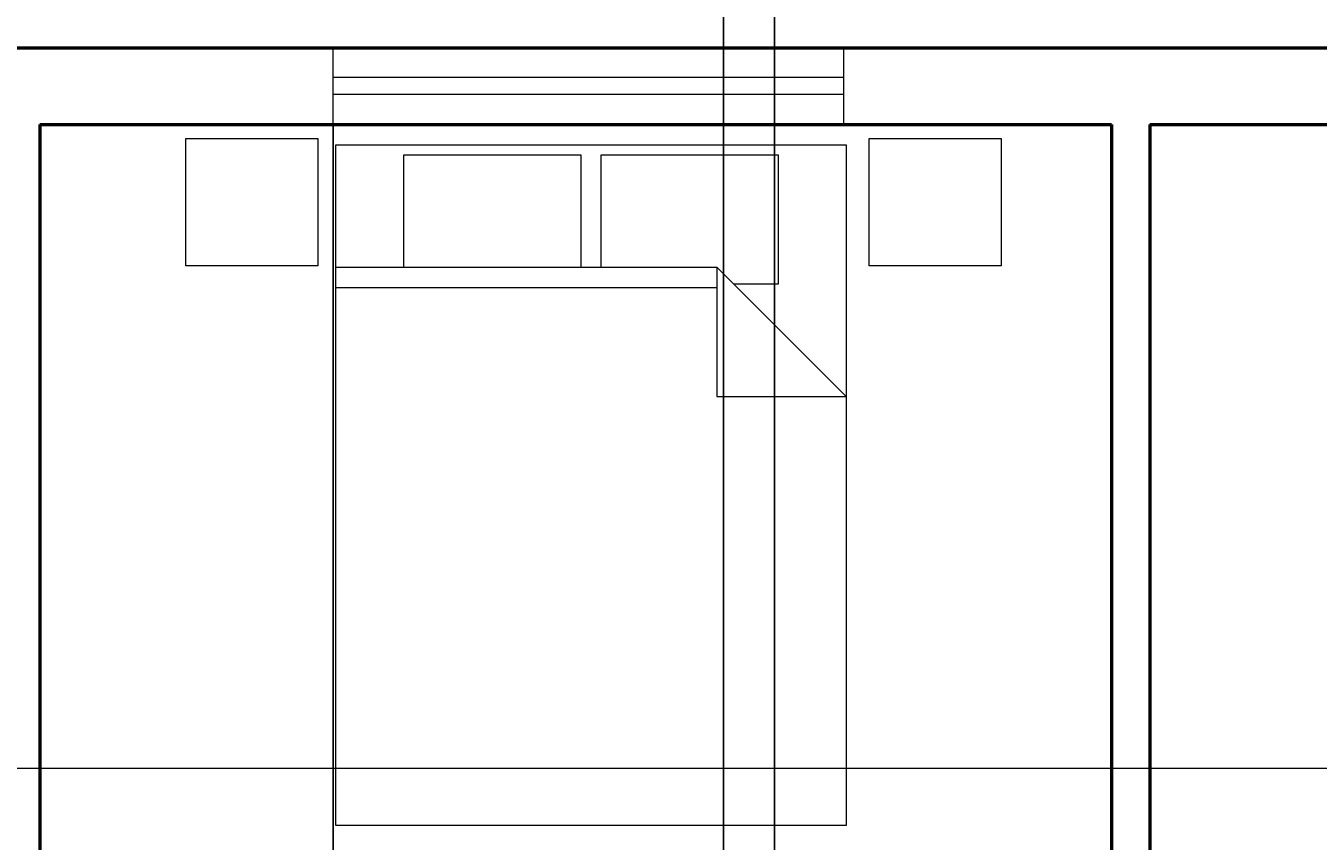
# Model space of a CAD drawing. Units: inches. Extents: x 7359 to 7979, y 33027 to 34263.
# Tile 16 of 32: x 7612 to 7764, y 33534 to 33630. Entities that reach past the tile are written whole.
import ezdxf

# ---------------------------------------------------------------- set-up
doc = ezdxf.new("R2010")
doc.units = ezdxf.units.IN
for name, color, linetype, lineweight in [('A-ANNO-DIMS', 2, 'Continuous', 18), ('A-ANNO-SYMB', 7, 'Continuous', 18), ('A-FURN', 8, 'Continuous', 18), ('A-GLAZ', 4, 'Continuous', 18), ('A-WALL', 7, 'Continuous', 50)]:
    doc.layers.add(name, color=color, linetype=linetype, lineweight=lineweight)
doc.styles.get("Standard").update_dxf_attribs({"font": 'arial.ttf'})
doc.dimstyles.get("Standard").update_dxf_attribs({"dimtxt": 0.18, "dimasz": 0.18, "dimexe": 0.18, "dimexo": 0.0625, "dimgap": 0.09, "dimtad": 0, "dimtih": 1, "dimtoh": 1, "dimdec": 4, "dimzin": 0, "dimdsep": 46, "dimtxsty": 'Standard', "dimcen": 0.09, "dimadec": 0, "dimazin": 0, "dimtfac": 1, "dimtdec": 4, "dimtofl": 0, "dimtmove": 0, "dimatfit": 3, "dimfxl": 1, "dimtolj": 1, "dimtzin": 0, "dimarcsym": 0})

# ---------------------------------------------------------------- blocks, each defined once
blk = doc.blocks.new('Bed - Queen')
for p, q in [((0, -80.00003), (0, 0)), ((0, 0), (59.99999, 0)), ((59.99999, 0), (59.99999, -80.00003)), ((7.99999, -1.2), (28.79998, -1.2)), ((7.99999, -14.4), (7.99999, -1.2)), ((28.79998, -1.2), (28.79998, -14.4)), ((31.19999, -1.2), (51.99999, -1.2)), ((31.19999, -14.4), (31.19999, -1.2)), ((51.99999, -1.2), (51.99999, -16.4)), ((0, -14.4), (44.8, -14.4)), ((59.99999, -29.6), (44.8, -14.4)), ((44.8, -14.4), (44.8, -29.6)), ((51.99999, -16.4), (46.79936, -16.4)), ((44.8, -16.8), (0, -16.8)), ((44.8, -29.6), (59.99999, -29.6)), ((59.99999, -80.00003), (0, -80.00003))]:
    blk.add_line(p, q)
blk = doc.blocks.new('TABLE-BEDSIDE')
blk.add_lwpolyline([(0, 15), (15.54, 15), (15.54, 0), (0, 0)], close=True)
blk = doc.blocks.new('WINDOW-W2-BEDROOM')
for p, q in [((0, 0), (0, 9)), ((60.05, 0), (60.05, 9)), ((60.05, 5.5), (0, 5.5)), ((60.05, 3.5), (0, 3.5))]:
    blk.add_line(p, q)
blk = doc.blocks.new('*D66')
at = {"layer": 'A-ANNO-DIMS', "color": 0, "lineweight": -2, "transparency": 16777216}
for p, q in [((7468.73, 33627.22), (7468.73, 33657.24)), ((7468.91, 33657.06), (7681.03, 33657.06)), ((7893.95, 33657.06), (7681.82, 33657.06)), ((7894.13, 33627.22), (7894.13, 33657.24))]:
    blk.add_line(p, q, dxfattribs=at)
at = {"layer": 'A-ANNO-DIMS', "color": 0, "transparency": 16777216}
for points in [[(7468.91, 33657.09), (7468.91, 33657.03), (7468.73, 33657.06)], [(7893.95, 33657.09), (7893.95, 33657.03), (7894.13, 33657.06)]]:
    blk.add_solid(points, dxfattribs=at)
at = {"layer": 'Defpoints', "color": 0, "transparency": 16777216}
for p in [(7894.13, 33657.06), (7468.73, 33627.16), (7894.13, 33627.16)]:
    blk.add_point(p, dxfattribs=at)
at = {"layer": 'A-ANNO-DIMS', "color": 0, "transparency": 16777216, "insert": (7681.43, 33657.06), "char_height": 0.18, "attachment_point": 5}
blk.add_mtext('\\A1;425.4', dxfattribs=at)
blk = doc.blocks.new('*D73')
at = {"layer": 'A-ANNO-DIMS', "color": 0, "lineweight": -2, "transparency": 16777216}
for p, q in [((7613.23, 33618.1), (7613.23, 33027.18)), ((7647.71, 33618.1), (7647.71, 33027.18)), ((7613.41, 33027.36), (7630.07, 33027.36)), ((7647.53, 33027.36), (7630.86, 33027.36))]:
    blk.add_line(p, q, dxfattribs=at)
at = {"layer": 'A-ANNO-DIMS', "color": 0, "transparency": 16777216}
for points in [[(7613.41, 33027.39), (7613.41, 33027.33), (7613.23, 33027.36)], [(7647.53, 33027.39), (7647.53, 33027.33), (7647.71, 33027.36)]]:
    blk.add_solid(points, dxfattribs=at)
at = {"layer": 'Defpoints', "color": 0, "transparency": 16777216}
for p in [(7613.23, 33618.16), (7647.71, 33618.16), (7647.71, 33027.36)]:
    blk.add_point(p, dxfattribs=at)
at = {"layer": 'A-ANNO-DIMS', "color": 0, "transparency": 16777216, "insert": (7630.47, 33027.36), "char_height": 0.18, "attachment_point": 5}
blk.add_mtext('\\A1;34.48', dxfattribs=at)
blk = doc.blocks.new('*D74')
at = {"layer": 'A-ANNO-DIMS', "color": 0, "lineweight": -2, "transparency": 16777216}
for p, q in [((7743.73, 33618.1), (7743.73, 33027.18)), ((7787.03, 33618.1), (7787.03, 33027.18)), ((7743.91, 33027.36), (7765, 33027.36)), ((7786.85, 33027.36), (7765.76, 33027.36))]:
    blk.add_line(p, q, dxfattribs=at)
at = {"layer": 'A-ANNO-DIMS', "color": 0, "transparency": 16777216}
for points in [[(7743.91, 33027.39), (7743.91, 33027.33), (7743.73, 33027.36)], [(7786.85, 33027.39), (7786.85, 33027.33), (7787.03, 33027.36)]]:
    blk.add_solid(points, dxfattribs=at)
at = {"layer": 'Defpoints', "color": 0, "transparency": 16777216}
for p in [(7743.73, 33618.16), (7787.03, 33618.16), (7787.03, 33027.36)]:
    blk.add_point(p, dxfattribs=at)
at = {"layer": 'A-ANNO-DIMS', "color": 0, "transparency": 16777216, "insert": (7765.38, 33027.36), "char_height": 0.18, "attachment_point": 5}
blk.add_mtext('\\A1;43.31', dxfattribs=at)
blk = doc.blocks.new('*D89')
at = {"layer": 'A-ANNO-DIMS', "color": 0, "lineweight": -2, "transparency": 16777216}
for p, q in [((7693.626578, 33301.124789), (7693.626578, 33657.242289)), ((7693.806578, 33657.062289), (7696.477151, 33657.062289)), ((7699.446578, 33657.062289), (7696.776005, 33657.062289)), ((7699.626578, 33301.124789), (7699.626578, 33657.242289))]:
    blk.add_line(p, q, dxfattribs=at)
at = {"layer": 'A-ANNO-DIMS', "color": 0, "transparency": 16777216}
for points in [[(7693.806578, 33657.092289), (7693.806578, 33657.032289), (7693.626578, 33657.062289)], [(7699.446578, 33657.092289), (7699.446578, 33657.032289), (7699.626578, 33657.062289)]]:
    blk.add_solid(points, dxfattribs=at)
at = {"layer": 'Defpoints', "color": 0, "transparency": 16777216}
for p in [(7699.626578, 33657.062289), (7693.626578, 33301.062289), (7699.626578, 33301.062289)]:
    blk.add_point(p, dxfattribs=at)
at = {"layer": 'A-ANNO-DIMS', "color": 0, "transparency": 16777216, "insert": (7696.626578, 33657.062289), "char_height": 0.18, "attachment_point": 5}
blk.add_mtext('\\A1;6', dxfattribs=at)

msp = doc.modelspace()

# ---------------------------------------------------------------- linework, layer by layer
at = {"layer": 'A-ANNO-SYMB'}
msp.add_line((7406.9423, 33542.482), (7940.6696, 33542.482), dxfattribs=at)
at = {"layer": 'A-WALL'}
for p, q in [((7468.7266, 33627.1623), (7894.1266, 33627.1623)), ((7613.2266, 33618.1623), (7739.2266, 33618.1623)), ((7613.2266, 33618.1623), (7613.2266, 33475.6623)), ((7739.2266, 33618.1623), (7739.2266, 33475.6623)), ((7743.7266, 33618.1623), (7885.1266, 33618.1623)), ((7743.7266, 33618.1623), (7743.7266, 33453.1623))]:
    msp.add_line(p, q, dxfattribs=at)

# ---------------------------------------------------------------- block references
at = {"layer": 'A-FURN'}
for name, p in [('TABLE-BEDSIDE', (7630.3961, 33601.5164)), ('Bed - Queen', (7648.0357, 33615.7623)), ('TABLE-BEDSIDE', (7710.7362, 33601.5164))]:
    msp.add_blockref(name, p, dxfattribs=at)
at = {"layer": 'A-GLAZ'}
msp.add_blockref('WINDOW-W2-BEDROOM', (7647.7061, 33618.1624), dxfattribs=at)

# ---------------------------------------------------------------- dimensions: what is measured, and where the dimension line sits
at = {"layer": 'A-ANNO-DIMS'}
for base, p1, p2, override, picture, middle in [((7894.1266, 33657.0623), (7468.7266, 33627.1623), (7894.1266, 33627.1623), {"dimdec": 1, "dimlfac": 1, "dimrnd": 0, "dimzin": 0, "dimdsep": 46, "dimlunit": 2}, '*D66', (7681.4266, 33657.0623)), ((7699.6266, 33657.0623), (7693.6266, 33301.0623), (7699.6266, 33301.0623), {"dimdec": 0, "dimlfac": 1, "dimrnd": 0, "dimzin": 0, "dimdsep": 46, "dimlunit": 2}, '*D89', (7696.6266, 33657.0623)), ((7647.7062, 33027.3568), (7613.2266, 33618.1623), (7647.7062, 33618.1623), {"dimdec": 2, "dimlfac": 1, "dimrnd": 0, "dimzin": 0, "dimdsep": 46, "dimlunit": 2}, '*D73', (7630.4664, 33027.3568)), ((7787.0342, 33027.3568), (7743.7266, 33618.1623), (7787.0342, 33618.1623), {"dimdec": 2, "dimlfac": 1, "dimrnd": 0, "dimzin": 0, "dimdsep": 46, "dimlunit": 2}, '*D74', (7765.3804, 33027.3568))]:
    dim = msp.add_linear_dim(base=base, p1=p1, p2=p2, dimstyle='Standard', override=override, dxfattribs=at)
    dim.commit()
    dim.dimension.update_dxf_attribs({"geometry": picture, "text_midpoint": middle})

doc.saveas('drawing.dxf')
